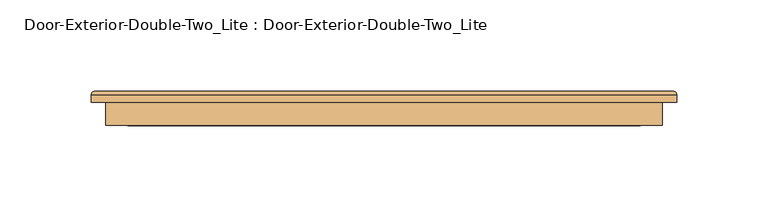
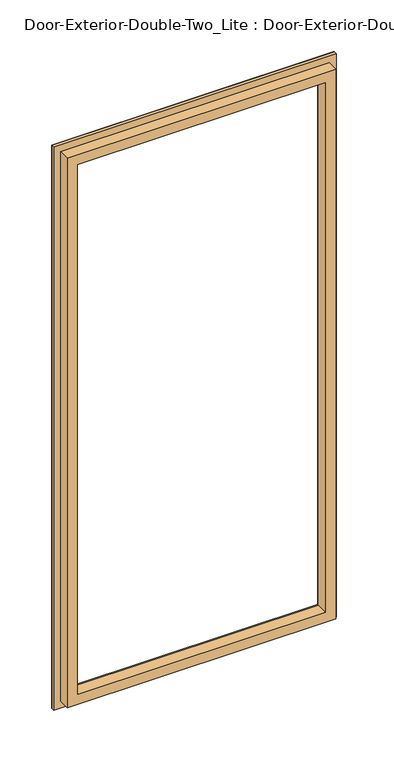
"""IFC4 building model written with IfcOpenShell, lengths in millimetres: door geometry, Door-Exterior-Double-Two_Lite : Door-Exterior-Double-Two_Lite."""

from ifc_helpers import new_model, si_unit, frame, origin, place, context, project, spatial, ellipse_curve, source, transform, mapped, element, save
from ifc_brep_helpers import plane_surface, cylinder_surface, advanced_brep


def door_exterior_double_two_lite_door_exterior_double_two_lite_4a402bc0(model_context):
    return source(origin(), model_context, "Body", "AdvancedBrep", [
        advanced_brep(
        [(-457.2, 82.55, 914.4), (-457.2, 95.25, 914.4), (-457.2, 95.25, 254.0), (-457.2, 82.55, 254.0), (-445.2, 96.25, 902.4), (-445.2, 82.55, 902.4), (-445.2, 82.55, 266.0), (-445.2, 96.25, 266.0), (-450.2, 101.25, 907.4), (-450.2, 101.25, 261.0), (-465.2, 99.25, 922.4), (-463.2, 101.25, 920.4), (-463.2, 101.25, 248.0), (-465.2, 99.25, 246.0), (-465.2, 95.25, 922.4), (-465.2, 95.25, 246.0), (-152.4, 95.25, 254.0), (-152.4, 82.55, 254.0), (-164.4, 82.55, 266.0), (-164.4, 96.25, 266.0), (-159.4, 101.25, 261.0), (-146.4, 101.25, 248.0), (-144.4, 99.25, 246.0), (-144.4, 95.25, 246.0), (-152.4, 95.25, 914.4), (-152.4, 82.55, 914.4), (-164.4, 82.55, 902.4), (-164.4, 96.25, 902.4), (-159.4, 101.25, 907.4), (-146.4, 101.25, 920.4), (-144.4, 99.25, 922.4), (-144.4, 95.25, 922.4)],
        [
            (0, 1),
            (1, 2),
            (2, 3),
            (3, 0),
            (4, 5),
            (5, 6),
            (6, 7),
            (7, 4),
            (8, 4, ellipse_curve(frame((-450.2, 96.25, 907.4), z_axis=(-0.7071067811865475, 0.0, -0.7071067811865475), x_axis=(-0.7071067811865474, 0.0, 0.7071067811865476)), 7.0710678, 5.0)),
            (7, 9, ellipse_curve(frame((-450.2, 96.25, 261.0), z_axis=(-0.7071067811865475, 0.0, 0.7071067811865475), x_axis=(0.7071067811865474, 0.0, 0.7071067811865476)), 7.0710678, 5.0)),
            (9, 8),
            (10, 11, ellipse_curve(frame((-463.2, 99.25, 920.4), z_axis=(-0.7071067811865475, 0.0, -0.7071067811865475), x_axis=(-0.7071067811865474, 0.0, 0.7071067811865476)), 2.8284271, 2.0)),
            (11, 12),
            (12, 13, ellipse_curve(frame((-463.2, 99.25, 248.0), z_axis=(-0.7071067811865475, 0.0, 0.7071067811865475), x_axis=(0.7071067811865474, 0.0, 0.7071067811865476)), 2.8284271, 2.0)),
            (13, 10),
            (14, 10),
            (13, 15),
            (15, 14),
            (2, 16),
            (16, 17),
            (17, 3),
            (6, 18),
            (18, 19),
            (19, 7),
            (19, 20, ellipse_curve(frame((-159.4, 96.25, 261.0), z_axis=(-0.7071067811865475, 0.0, -0.7071067811865475), x_axis=(-0.7071067811865476, 0.0, 0.7071067811865474)), 7.0710678, 5.0)),
            (20, 9),
            (12, 21),
            (21, 22, ellipse_curve(frame((-146.4, 99.25, 248.0), z_axis=(-0.7071067811865475, 0.0, -0.7071067811865475), x_axis=(-0.7071067811865476, 0.0, 0.7071067811865474)), 2.8284271, 2.0)),
            (22, 13),
            (22, 23),
            (23, 15),
            (16, 24),
            (24, 25),
            (25, 17),
            (18, 26),
            (26, 27),
            (27, 19),
            (27, 28, ellipse_curve(frame((-159.4, 96.25, 907.4), z_axis=(0.7071067811865475, 0.0, -0.7071067811865475), x_axis=(-0.7071067811865474, 0.0, -0.7071067811865476)), 7.0710678, 5.0)),
            (28, 20),
            (21, 29),
            (29, 30, ellipse_curve(frame((-146.4, 99.25, 920.4), z_axis=(0.7071067811865475, 0.0, -0.7071067811865475), x_axis=(-0.7071067811865474, 0.0, -0.7071067811865476)), 2.8284271, 2.0)),
            (30, 22),
            (30, 31),
            (31, 23),
            (31, 14),
            (1, 24),
            (0, 25),
            (5, 26),
            (4, 27),
            (8, 28),
            (11, 29),
            (10, 30),
        ],
        [
            plane_surface(frame((-457.2, 95.25, 914.4), z_axis=(-1.0, 0.0, 0.0), x_axis=(0.0, 0.0, -1.0))),
            plane_surface(frame((-445.2, 82.55, 902.4), z_axis=(1.0, 0.0, 0.0), x_axis=(0.0, 0.0, -1.0))),
            cylinder_surface(frame((-450.2, 96.25, 914.4), z_axis=(0.0, 0.0, 1.0), x_axis=(-1.0, 0.0, 0.0)), 5.0),
            cylinder_surface(frame((-463.2, 99.25, 914.4), z_axis=(0.0, 0.0, 1.0), x_axis=(-1.0, 0.0, 0.0)), 2.0),
            plane_surface(frame((-465.2, 99.25, 922.4), z_axis=(-1.0, 0.0, 0.0), x_axis=(0.0, 0.0, -1.0))),
            plane_surface(frame((-457.2, 95.25, 254.0), z_axis=(0.0, 0.0, -1.0), x_axis=(1.0, 0.0, 0.0))),
            plane_surface(frame((-445.2, 82.55, 266.0), z_axis=(0.0, 0.0, 1.0), x_axis=(1.0, 0.0, 0.0))),
            cylinder_surface(frame((-457.2, 96.25, 261.0), z_axis=(-1.0, 0.0, 0.0), x_axis=(0.0, 0.0, -1.0)), 5.0),
            cylinder_surface(frame((-457.2, 99.25, 248.0), z_axis=(-1.0, 0.0, 0.0), x_axis=(0.0, 0.0, -1.0)), 2.0),
            plane_surface(frame((-465.2, 99.25, 246.0), z_axis=(0.0, 0.0, -1.0), x_axis=(1.0, 0.0, 0.0))),
            plane_surface(frame((-152.4, 95.25, 254.0), z_axis=(1.0, 0.0, 0.0), x_axis=(0.0, 0.0, 1.0))),
            plane_surface(frame((-164.4, 82.55, 266.0), z_axis=(-1.0, 0.0, 0.0), x_axis=(0.0, 0.0, 1.0))),
            cylinder_surface(frame((-159.4, 96.25, 254.0), z_axis=(0.0, 0.0, -1.0), x_axis=(1.0, 0.0, 0.0)), 5.0),
            cylinder_surface(frame((-146.4, 99.25, 254.0), z_axis=(0.0, 0.0, -1.0), x_axis=(1.0, 0.0, 0.0)), 2.0),
            plane_surface(frame((-144.4, 99.25, 246.0), z_axis=(1.0, 0.0, 0.0), x_axis=(0.0, 0.0, 1.0))),
            plane_surface(frame((-144.4, 95.25, 922.4), z_axis=(0.0, -1.0, 0.0), x_axis=(-1.0, 0.0, 0.0))),
            plane_surface(frame((-152.4, 95.25, 914.4), z_axis=(0.0, 0.0, 1.0), x_axis=(-1.0, 0.0, 0.0))),
            plane_surface(frame((-152.4, 82.55, 914.4), z_axis=(0.0, -1.0, 0.0), x_axis=(-1.0, 0.0, 0.0))),
            plane_surface(frame((-164.4, 82.55, 902.4), z_axis=(0.0, 0.0, -1.0), x_axis=(-1.0, 0.0, 0.0))),
            cylinder_surface(frame((-152.4, 96.25, 907.4), z_axis=(1.0, 0.0, 0.0), x_axis=(0.0, 0.0, 1.0)), 5.0),
            plane_surface(frame((-159.4, 101.25, 907.4), z_axis=(0.0, 1.0, 0.0), x_axis=(-1.0, 0.0, 0.0))),
            cylinder_surface(frame((-152.4, 99.25, 920.4), z_axis=(1.0, 0.0, 0.0), x_axis=(0.0, 0.0, 1.0)), 2.0),
            plane_surface(frame((-144.4, 99.25, 922.4), z_axis=(0.0, 0.0, 1.0), x_axis=(-1.0, 0.0, 0.0))),
        ],
        [
            (0, [[1, 2, 3, 4]]),
            (1, [[5, 6, 7, 8]]),
            (2, [[9, -8, 10, 11]]),
            (3, [[12, 13, 14, 15]]),
            (4, [[16, -15, 17, 18]]),
            (5, [[-3, 19, 20, 21]]),
            (6, [[-7, 22, 23, 24]]),
            (7, [[-10, -24, 25, 26]]),
            (8, [[-14, 27, 28, 29]]),
            (9, [[-17, -29, 30, 31]]),
            (10, [[-20, 32, 33, 34]]),
            (11, [[-23, 35, 36, 37]]),
            (12, [[-25, -37, 38, 39]]),
            (13, [[-28, 40, 41, 42]]),
            (14, [[-30, -42, 43, 44]]),
            (15, [[-31, -44, 45, -18], [46, -32, -19, -2]]),
            (16, [[-33, -46, -1, 47]]),
            (17, [[-21, -34, -47, -4], [48, -35, -22, -6]]),
            (18, [[-36, -48, -5, 49]]),
            (19, [[-38, -49, -9, 50]]),
            (20, [[51, -40, -27, -13], [-26, -39, -50, -11]]),
            (21, [[-41, -51, -12, 52]]),
            (22, [[-43, -52, -16, -45]]),
        ],
    ),
    ])


if __name__ == "__main__":
    model = new_model("IFC4")
    model_context = context("Model", 3, world=origin())
    ifc_project = project(units=[si_unit("LENGTHUNIT", "METRE", prefix="MILLI")], contexts=[model_context])
    site = spatial("IfcSite", under=ifc_project)
    building = spatial("IfcBuilding", under=site)
    placement = place(None, origin())
    door_exterior_double_two_lite_door_exterior_double_two_lite_shape = door_exterior_double_two_lite_door_exterior_double_two_lite_4a402bc0(model_context)
    element("IfcDoor", 1, ObjectType="Door-Exterior-Double-Two_Lite : Door-Exterior-Double-Two_Lite", at=placement, inside=building, context=model_context, shape_type="MappedRepresentation", body=[
        mapped(door_exterior_double_two_lite_door_exterior_double_two_lite_shape, transform((0.0, 0.0, 0.0), x_axis=(1.0, 0.0, 0.0), y_axis=(0.0, 1.0, 0.0), z_axis=(0.0, 0.0, 1.0))),
    ])
    save(model, "model.ifc")

# Revit data of these elements
# Type "Door-Exterior-Double-Two_Lite : Door-Exterior-Double-Two_Lite"
#   Type Mark = "8"
#   Assembly Code = "B2030100"
#   Analytic Construction = "Metal frame, double glass door"
#   Top Rail = 0' - 4 5/8"
#   Threshold Length [instance default] = 4' - 4"
#   Threshold Offset [instance default] = 0' - 0 1/2"
#   Thickness = 0' - 1 3/4"
#   Thermal Resistance (R) = 1.3794 (h·ft²·°F)/BTU
#   Swing Angle [instance default] = 90.00°
#   Strike Height = 3' - 4"
#   Stiles = 0' - 6"
#   SinglePanelWidth = 2' - 0"
#   Rough Width [instance default] = 4' - 4"
#   Rough Height [instance default] = 7' - 4"
#   MFOpeningHeight [instance default] = 0' - 4"
#   MFOpeningWidth [instance default] = 0' - 4"
#   Lock Rail = 0' - 8"
#   Inset Calculate [instance default] = 0' - 4"
#   Masonry Inset [instance default] = 0' - 1"
#   Height = 7' - 0"
#   Width = 4' - 0"
#   Heat Transfer Coefficient (U) = 0.7250 BTU/(h·ft²·°F)
#   Glass Thickness = 0' - 0 3/4"
#   Masonry Frame Depth = 0' - 5 3/4"
#   Bottom Rail = 0' - 10"
#   Threshold [instance default] = yes
#   Masonry Frame [instance default] = yes
#   Function = 1
#   Dry Wall Frame [instance default] = no
#   Threshold Material = none
#   Panic Bar Material = Metal - Stainless Steel
#   Panel Material = Metal - Painted - Grey
#   Glass Stop Material = Metal - Painted - Grey
#   Frame Material = Metal - Painted - Grey
#   Exterior Pull Material = Metal - Stainless Steel
#   Visual Light Transmittance = 0
#   Solar Heat Gain Coefficient = 0
#   Wall Closure = (empty or 0)
# Element 1 (IfcDoor, "Door-Exterior-Double-Two_Lite : Door-Exterior-Double-Two_Lite")
#   Materials on its faces: "Metal - Painted - Grey", "Metal - Stainless Steel", "Glass"
# Materials
#   "Metal - Stainless Steel": class "Metal", colour RGB 247 247 247, transparency 0
#   "Metal - Painted - Grey": class "Paint", colour RGB 104 104 104, transparency 0, Cost = 0
#   "Glass": class "Glass", colour RGB 0 128 192, transparency 0.75, Description = "Soda Lime Glass", Cost = 0
